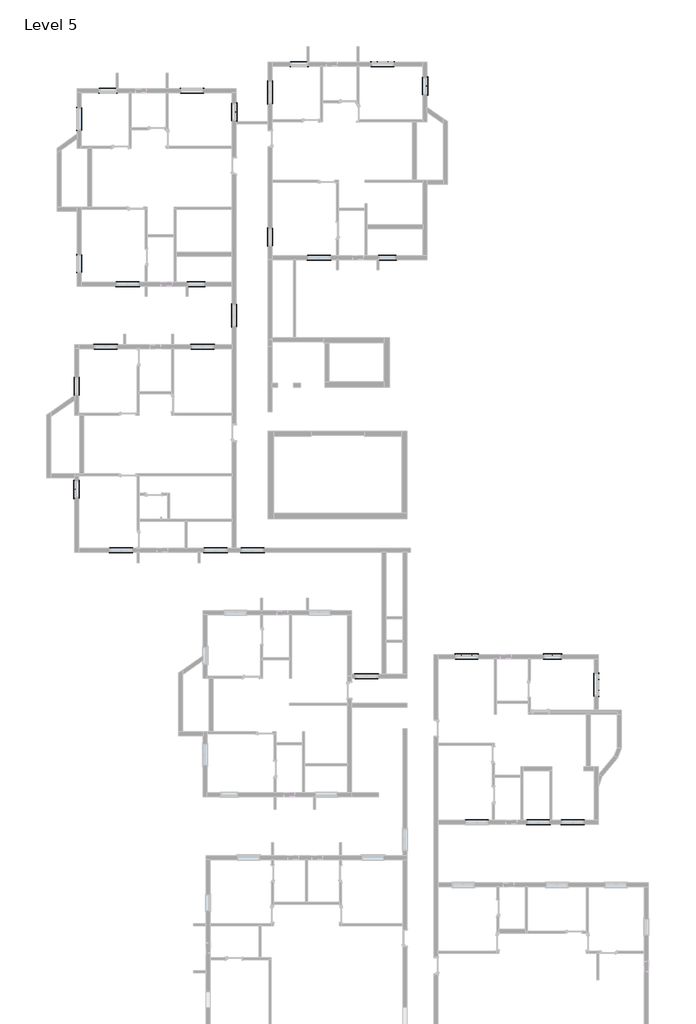
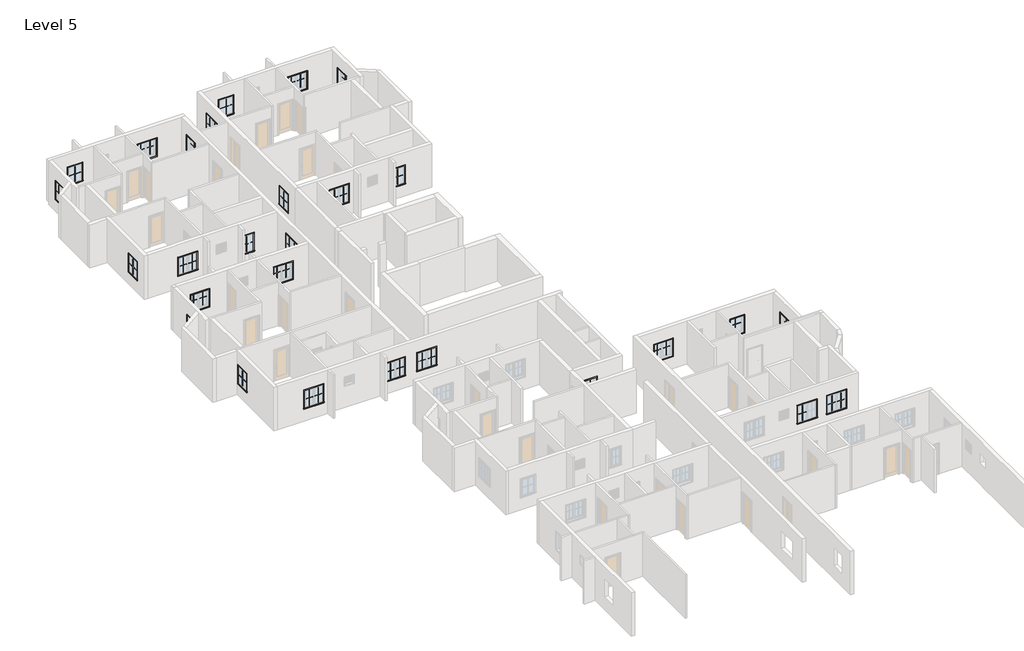
# One storey, part 7 of 7: 101 proxies.
"""IFC4 building model written with IfcOpenShell, lengths in millimetres."""

from ifc_helpers import new_model, si_unit, origin, place, context, project, spatial, transform, mapped, element, save
from components import muntin_pattern_2x2_muntin_pattern_2x2_95b57395, muntin_pattern_2x2_muntin_pattern_2x2_4dfeb3f3, muntin_pattern_2x2_muntin_pattern_2x2_e852a7e4, trim_window_exterior_flat_with_sill_e4b28ec3, trim_window_exterior_flat_with_sill_7cfdd449, trim_window_interior_flat_picture_frame_39ff4276, trim_window_interior_flat_picture_frame_f1e0b15b

model = new_model("IFC4")

# Units and contexts
model_context = context("Model", 3, world=origin())
ifc_project = project(units=[si_unit("LENGTHUNIT", "METRE", prefix="MILLI")], contexts=[model_context])

# Site, building, storey
site = spatial("IfcSite", under=ifc_project)
building = spatial("IfcBuilding", under=site)
storey = spatial("IfcBuildingStorey", under=building, Name="Level 5", Elevation=6400.8)

# Proxies
placement = place(None, origin())
muntin_pattern_2x2_muntin_pattern_2x2_shape = muntin_pattern_2x2_muntin_pattern_2x2_95b57395(model_context)
element("IfcBuildingElementProxy", 1, Name="Muntin Pattern_2x2 : Muntin Pattern_2x2", ObjectType="Muntin Pattern_2x2 : Muntin Pattern_2x2", at=placement, inside=storey, context=model_context, shape_type="MappedRepresentation", body=[
    mapped(muntin_pattern_2x2_muntin_pattern_2x2_shape, transform((-14884.6759469, 4921.5461172, 7385.05), x_axis=(0.0, 1.0, 0.0), y_axis=(-1.0, 0.0, 0.0), z_axis=(0.0, 0.0, 1.0))),
])
element("IfcBuildingElementProxy", 2, Name="Muntin Pattern_2x2 : Muntin Pattern_2x2", ObjectType="Muntin Pattern_2x2 : Muntin Pattern_2x2", at=placement, inside=storey, context=model_context, shape_type="MappedRepresentation", body=[
    mapped(muntin_pattern_2x2_muntin_pattern_2x2_shape, transform((-12990.7362554, 27537.0711172, 7385.05), x_axis=(-1.0, 0.0, 0.0), y_axis=(0.0, -1.0, 0.0), z_axis=(0.0, 0.0, 1.0))),
])
element("IfcBuildingElementProxy", 3, Name="Muntin Pattern_2x2 : Muntin Pattern_2x2", ObjectType="Muntin Pattern_2x2 : Muntin Pattern_2x2", at=placement, inside=storey, context=model_context, shape_type="MappedRepresentation", body=[
    mapped(muntin_pattern_2x2_muntin_pattern_2x2_shape, transform((-5683.5259469, 26431.1755084, 7385.05), x_axis=(0.0, -1.0, 0.0), y_axis=(1.0, 0.0, 0.0), z_axis=(0.0, 0.0, 1.0))),
])
element("IfcBuildingElementProxy", 4, Name="Muntin Pattern_2x2 : Muntin Pattern_2x2", ObjectType="Muntin Pattern_2x2 : Muntin Pattern_2x2", at=placement, inside=storey, context=model_context, shape_type="MappedRepresentation", body=[
    mapped(muntin_pattern_2x2_muntin_pattern_2x2_shape, transform((-7960.0009469, 16513.4711172, 7385.05), x_axis=(-1.0, 0.0, 0.0), y_axis=(0.0, -1.0, 0.0), z_axis=(0.0, 0.0, 1.0))),
])
element("IfcBuildingElementProxy", 5, Name="Muntin Pattern_2x2 : Muntin Pattern_2x2", ObjectType="Muntin Pattern_2x2 : Muntin Pattern_2x2", at=placement, inside=storey, context=model_context, shape_type="MappedRepresentation", body=[
    mapped(muntin_pattern_2x2_muntin_pattern_2x2_shape, transform((-14732.2759469, 17786.6461172, 7385.05), x_axis=(0.0, 1.0, 0.0), y_axis=(-1.0, 0.0, 0.0), z_axis=(0.0, 0.0, 1.0))),
])
element("IfcBuildingElementProxy", 6, Name="Muntin Pattern_2x2 : Muntin Pattern_2x2", ObjectType="Muntin Pattern_2x2 : Muntin Pattern_2x2", at=placement, inside=storey, context=model_context, shape_type="MappedRepresentation", body=[
    mapped(muntin_pattern_2x2_muntin_pattern_2x2_shape, transform((-2075.0862554, 29050.5505084, 7385.05), x_axis=(-1.0, 0.0, 0.0), y_axis=(0.0, -1.0, 0.0), z_axis=(0.0, 0.0, 1.0))),
])
element("IfcBuildingElementProxy", 7, Name="Muntin Pattern_2x2 : Muntin Pattern_2x2", ObjectType="Muntin Pattern_2x2 : Muntin Pattern_2x2", at=placement, inside=storey, context=model_context, shape_type="MappedRepresentation", body=[
    mapped(muntin_pattern_2x2_muntin_pattern_2x2_shape, transform((5213.0740531, 27910.7255084, 7385.05), x_axis=(0.0, -1.0, 0.0), y_axis=(1.0, 0.0, 0.0), z_axis=(0.0, 0.0, 1.0))),
])
element("IfcBuildingElementProxy", 8, Name="Muntin Pattern_2x2 : Muntin Pattern_2x2", ObjectType="Muntin Pattern_2x2 : Muntin Pattern_2x2", at=placement, inside=storey, context=model_context, shape_type="MappedRepresentation", body=[
    mapped(muntin_pattern_2x2_muntin_pattern_2x2_shape, transform((2936.5990531, 18026.9505084, 7385.05), x_axis=(-1.0, 0.0, 0.0), y_axis=(0.0, -1.0, 0.0), z_axis=(0.0, 0.0, 1.0))),
])
element("IfcBuildingElementProxy", 9, Name="Muntin Pattern_2x2 : Muntin Pattern_2x2", ObjectType="Muntin Pattern_2x2 : Muntin Pattern_2x2", at=placement, inside=storey, context=model_context, shape_type="MappedRepresentation", body=[
    mapped(muntin_pattern_2x2_muntin_pattern_2x2_shape, transform((-3835.6759469, 19300.1255084, 7385.05), x_axis=(0.0, 1.0, 0.0), y_axis=(-1.0, 0.0, 0.0), z_axis=(0.0, 0.0, 1.0))),
])
element("IfcBuildingElementProxy", 10, Name="Muntin Pattern_2x2 : Muntin Pattern_2x2", ObjectType="Muntin Pattern_2x2 : Muntin Pattern_2x2", at=placement, inside=storey, context=model_context, shape_type="MappedRepresentation", body=[
    mapped(muntin_pattern_2x2_muntin_pattern_2x2_shape, transform((12366.3490531, -4512.6747229, 7385.05), x_axis=(1.0, 0.0, 0.0), y_axis=(0.0, 1.0, 0.0), z_axis=(0.0, 0.0, 1.0))),
])
element("IfcBuildingElementProxy", 11, Name="Muntin Pattern_2x2 : Muntin Pattern_2x2", ObjectType="Muntin Pattern_2x2 : Muntin Pattern_2x2", at=placement, inside=storey, context=model_context, shape_type="MappedRepresentation", body=[
    mapped(muntin_pattern_2x2_muntin_pattern_2x2_shape, transform((-14675.1259469, 10795.2961172, 7385.05), x_axis=(0.0, -1.0, 0.0), y_axis=(1.0, 0.0, 0.0), z_axis=(0.0, 0.0, 1.0))),
])
muntin_pattern_2x2_muntin_pattern_2x2_2_shape = muntin_pattern_2x2_muntin_pattern_2x2_4dfeb3f3(model_context)
element("IfcBuildingElementProxy", 12, Name="Muntin Pattern_2x2 : Muntin Pattern_2x2", ObjectType="Muntin Pattern_2x2 : Muntin Pattern_2x2", at=placement, inside=storey, context=model_context, shape_type="MappedRepresentation", body=[
    mapped(muntin_pattern_2x2_muntin_pattern_2x2_2_shape, transform((-8498.1634469, 27746.6211172, 7385.05), x_axis=(1.0, 0.0, 0.0), y_axis=(0.0, 1.0, 0.0), z_axis=(0.0, 0.0, 1.0))),
])
element("IfcBuildingElementProxy", 13, Name="Muntin Pattern_2x2 : Muntin Pattern_2x2", ObjectType="Muntin Pattern_2x2 : Muntin Pattern_2x2", at=placement, inside=storey, context=model_context, shape_type="MappedRepresentation", body=[
    mapped(muntin_pattern_2x2_muntin_pattern_2x2_2_shape, transform((-14732.2759469, 25728.9086172, 7385.05), x_axis=(0.0, 1.0, 0.0), y_axis=(-1.0, 0.0, 0.0), z_axis=(0.0, 0.0, 1.0))),
])
element("IfcBuildingElementProxy", 14, Name="Muntin Pattern_2x2 : Muntin Pattern_2x2", ObjectType="Muntin Pattern_2x2 : Muntin Pattern_2x2", at=placement, inside=storey, context=model_context, shape_type="MappedRepresentation", body=[
    mapped(muntin_pattern_2x2_muntin_pattern_2x2_2_shape, transform((-11562.0384469, 16513.4711172, 7385.05), x_axis=(-1.0, 0.0, 0.0), y_axis=(0.0, -1.0, 0.0), z_axis=(0.0, 0.0, 1.0))),
])
element("IfcBuildingElementProxy", 15, Name="Muntin Pattern_2x2 : Muntin Pattern_2x2", ObjectType="Muntin Pattern_2x2 : Muntin Pattern_2x2", at=placement, inside=storey, context=model_context, shape_type="MappedRepresentation", body=[
    mapped(muntin_pattern_2x2_muntin_pattern_2x2_2_shape, transform((-3835.6759469, 27242.3880084, 7385.05), x_axis=(0.0, 1.0, 0.0), y_axis=(-1.0, 0.0, 0.0), z_axis=(0.0, 0.0, 1.0))),
])
element("IfcBuildingElementProxy", 16, Name="Muntin Pattern_2x2 : Muntin Pattern_2x2", ObjectType="Muntin Pattern_2x2 : Muntin Pattern_2x2", at=placement, inside=storey, context=model_context, shape_type="MappedRepresentation", body=[
    mapped(muntin_pattern_2x2_muntin_pattern_2x2_2_shape, transform((2373.0365531, 29260.1005084, 7385.05), x_axis=(1.0, 0.0, 0.0), y_axis=(0.0, 1.0, 0.0), z_axis=(0.0, 0.0, 1.0))),
])
element("IfcBuildingElementProxy", 17, Name="Muntin Pattern_2x2 : Muntin Pattern_2x2", ObjectType="Muntin Pattern_2x2 : Muntin Pattern_2x2", at=placement, inside=storey, context=model_context, shape_type="MappedRepresentation", body=[
    mapped(muntin_pattern_2x2_muntin_pattern_2x2_2_shape, transform((-640.0384469, 18026.9505084, 7385.05), x_axis=(-1.0, 0.0, 0.0), y_axis=(0.0, -1.0, 0.0), z_axis=(0.0, 0.0, 1.0))),
])
element("IfcBuildingElementProxy", 18, Name="Muntin Pattern_2x2 : Muntin Pattern_2x2", ObjectType="Muntin Pattern_2x2 : Muntin Pattern_2x2", at=placement, inside=storey, context=model_context, shape_type="MappedRepresentation", body=[
    mapped(muntin_pattern_2x2_muntin_pattern_2x2_2_shape, transform((14979.3740531, -5923.9622229, 7385.05), x_axis=(0.0, -1.0, 0.0), y_axis=(1.0, 0.0, 0.0), z_axis=(0.0, 0.0, 1.0))),
])
element("IfcBuildingElementProxy", 19, Name="Muntin Pattern_2x2 : Muntin Pattern_2x2", ObjectType="Muntin Pattern_2x2 : Muntin Pattern_2x2", at=placement, inside=storey, context=model_context, shape_type="MappedRepresentation", body=[
    mapped(muntin_pattern_2x2_muntin_pattern_2x2_2_shape, transform((7173.6365531, -4512.6747229, 7385.05), x_axis=(1.0, 0.0, 0.0), y_axis=(0.0, 1.0, 0.0), z_axis=(0.0, 0.0, 1.0))),
])
element("IfcBuildingElementProxy", 20, Name="Muntin Pattern_2x2 : Muntin Pattern_2x2", ObjectType="Muntin Pattern_2x2 : Muntin Pattern_2x2", at=placement, inside=storey, context=model_context, shape_type="MappedRepresentation", body=[
    mapped(muntin_pattern_2x2_muntin_pattern_2x2_2_shape, transform((13825.2615531, -14158.3247229, 7385.05), x_axis=(-1.0, 0.0, 0.0), y_axis=(0.0, -1.0, 0.0), z_axis=(0.0, 0.0, 1.0))),
])
element("IfcBuildingElementProxy", 21, Name="Muntin Pattern_2x2 : Muntin Pattern_2x2", ObjectType="Muntin Pattern_2x2 : Muntin Pattern_2x2", at=placement, inside=storey, context=model_context, shape_type="MappedRepresentation", body=[
    mapped(muntin_pattern_2x2_muntin_pattern_2x2_2_shape, transform((1464.9865531, -5641.6788828, 7385.05), x_axis=(1.0, 0.0, 0.0), y_axis=(0.0, 1.0, 0.0), z_axis=(0.0, 0.0, 1.0))),
])
element("IfcBuildingElementProxy", 22, Name="Muntin Pattern_2x2 : Muntin Pattern_2x2", ObjectType="Muntin Pattern_2x2 : Muntin Pattern_2x2", at=placement, inside=storey, context=model_context, shape_type="MappedRepresentation", body=[
    mapped(muntin_pattern_2x2_muntin_pattern_2x2_2_shape, transform((-4443.6884469, 1349.6711172, 7385.05), x_axis=(-1.0, 0.0, 0.0), y_axis=(0.0, -1.0, 0.0), z_axis=(0.0, 0.0, 1.0))),
])
element("IfcBuildingElementProxy", 23, Name="Muntin Pattern_2x2 : Muntin Pattern_2x2", ObjectType="Muntin Pattern_2x2 : Muntin Pattern_2x2", at=placement, inside=storey, context=model_context, shape_type="MappedRepresentation", body=[
    mapped(muntin_pattern_2x2_muntin_pattern_2x2_2_shape, transform((-6540.8708092, 1349.6711172, 7385.05), x_axis=(-1.0, 0.0, 0.0), y_axis=(0.0, -1.0, 0.0), z_axis=(0.0, 0.0, 1.0))),
])
element("IfcBuildingElementProxy", 24, Name="Muntin Pattern_2x2 : Muntin Pattern_2x2", ObjectType="Muntin Pattern_2x2 : Muntin Pattern_2x2", at=placement, inside=storey, context=model_context, shape_type="MappedRepresentation", body=[
    mapped(muntin_pattern_2x2_muntin_pattern_2x2_2_shape, transform((-11943.0384469, 1349.6711172, 7385.05), x_axis=(-1.0, 0.0, 0.0), y_axis=(0.0, -1.0, 0.0), z_axis=(0.0, 0.0, 1.0))),
])
element("IfcBuildingElementProxy", 25, Name="Muntin Pattern_2x2 : Muntin Pattern_2x2", ObjectType="Muntin Pattern_2x2 : Muntin Pattern_2x2", at=placement, inside=storey, context=model_context, shape_type="MappedRepresentation", body=[
    mapped(muntin_pattern_2x2_muntin_pattern_2x2_2_shape, transform((-13424.2323258, 13141.6211172, 7385.05), x_axis=(1.0, 0.0, 0.0), y_axis=(0.0, 1.0, 0.0), z_axis=(0.0, 0.0, 1.0))),
])
element("IfcBuildingElementProxy", 26, Name="Muntin Pattern_2x2 : Muntin Pattern_2x2", ObjectType="Muntin Pattern_2x2 : Muntin Pattern_2x2", at=placement, inside=storey, context=model_context, shape_type="MappedRepresentation", body=[
    mapped(muntin_pattern_2x2_muntin_pattern_2x2_2_shape, transform((-7888.5634469, 13141.6211172, 7385.05), x_axis=(1.0, 0.0, 0.0), y_axis=(0.0, 1.0, 0.0), z_axis=(0.0, 0.0, 1.0))),
])
element("IfcBuildingElementProxy", 27, Name="Muntin Pattern_2x2 : Muntin Pattern_2x2", ObjectType="Muntin Pattern_2x2 : Muntin Pattern_2x2", at=placement, inside=storey, context=model_context, shape_type="MappedRepresentation", body=[
    mapped(muntin_pattern_2x2_muntin_pattern_2x2_2_shape, transform((-5893.0759469, 14524.3336172, 7385.05), x_axis=(0.0, 1.0, 0.0), y_axis=(-1.0, 0.0, 0.0), z_axis=(0.0, 0.0, 1.0))),
])
muntin_pattern_2x2_muntin_pattern_2x2_3_shape = muntin_pattern_2x2_muntin_pattern_2x2_e852a7e4(model_context)
element("IfcBuildingElementProxy", 28, Name="Muntin Pattern_2x2 : Muntin Pattern_2x2", ObjectType="Muntin Pattern_2x2 : Muntin Pattern_2x2", at=placement, inside=storey, context=model_context, shape_type="MappedRepresentation", body=[
    mapped(muntin_pattern_2x2_muntin_pattern_2x2_3_shape, transform((-7891.7384469, 27746.6211172, 7385.05), x_axis=(-1.0, 0.0, 0.0), y_axis=(0.0, -1.0, 0.0), z_axis=(0.0, 0.0, 1.0))),
])
element("IfcBuildingElementProxy", 29, Name="Muntin Pattern_2x2 : Muntin Pattern_2x2", ObjectType="Muntin Pattern_2x2 : Muntin Pattern_2x2", at=placement, inside=storey, context=model_context, shape_type="MappedRepresentation", body=[
    mapped(muntin_pattern_2x2_muntin_pattern_2x2_3_shape, transform((-14732.2759469, 26335.3336172, 7385.05), x_axis=(0.0, -1.0, 0.0), y_axis=(1.0, 0.0, 0.0), z_axis=(0.0, 0.0, 1.0))),
])
element("IfcBuildingElementProxy", 30, Name="Muntin Pattern_2x2 : Muntin Pattern_2x2", ObjectType="Muntin Pattern_2x2 : Muntin Pattern_2x2", at=placement, inside=storey, context=model_context, shape_type="MappedRepresentation", body=[
    mapped(muntin_pattern_2x2_muntin_pattern_2x2_3_shape, transform((-12168.4634469, 16513.4711172, 7385.05), x_axis=(1.0, 0.0, 0.0), y_axis=(0.0, 1.0, 0.0), z_axis=(0.0, 0.0, 1.0))),
])
element("IfcBuildingElementProxy", 31, Name="Muntin Pattern_2x2 : Muntin Pattern_2x2", ObjectType="Muntin Pattern_2x2 : Muntin Pattern_2x2", at=placement, inside=storey, context=model_context, shape_type="MappedRepresentation", body=[
    mapped(muntin_pattern_2x2_muntin_pattern_2x2_3_shape, transform((-3835.6759469, 27848.8130084, 7385.05), x_axis=(0.0, -1.0, 0.0), y_axis=(1.0, 0.0, 0.0), z_axis=(0.0, 0.0, 1.0))),
])
element("IfcBuildingElementProxy", 32, Name="Muntin Pattern_2x2 : Muntin Pattern_2x2", ObjectType="Muntin Pattern_2x2 : Muntin Pattern_2x2", at=placement, inside=storey, context=model_context, shape_type="MappedRepresentation", body=[
    mapped(muntin_pattern_2x2_muntin_pattern_2x2_3_shape, transform((2979.4615531, 29260.1005084, 7385.05), x_axis=(-1.0, 0.0, 0.0), y_axis=(0.0, -1.0, 0.0), z_axis=(0.0, 0.0, 1.0))),
])
element("IfcBuildingElementProxy", 33, Name="Muntin Pattern_2x2 : Muntin Pattern_2x2", ObjectType="Muntin Pattern_2x2 : Muntin Pattern_2x2", at=placement, inside=storey, context=model_context, shape_type="MappedRepresentation", body=[
    mapped(muntin_pattern_2x2_muntin_pattern_2x2_3_shape, transform((-1246.4634469, 18026.9505084, 7385.05), x_axis=(1.0, 0.0, 0.0), y_axis=(0.0, 1.0, 0.0), z_axis=(0.0, 0.0, 1.0))),
])
element("IfcBuildingElementProxy", 34, Name="Muntin Pattern_2x2 : Muntin Pattern_2x2", ObjectType="Muntin Pattern_2x2 : Muntin Pattern_2x2", at=placement, inside=storey, context=model_context, shape_type="MappedRepresentation", body=[
    mapped(muntin_pattern_2x2_muntin_pattern_2x2_3_shape, transform((14979.3740531, -6530.3872229, 7385.05), x_axis=(0.0, 1.0, 0.0), y_axis=(-1.0, 0.0, 0.0), z_axis=(0.0, 0.0, 1.0))),
])
element("IfcBuildingElementProxy", 35, Name="Muntin Pattern_2x2 : Muntin Pattern_2x2", ObjectType="Muntin Pattern_2x2 : Muntin Pattern_2x2", at=placement, inside=storey, context=model_context, shape_type="MappedRepresentation", body=[
    mapped(muntin_pattern_2x2_muntin_pattern_2x2_3_shape, transform((7780.0615531, -4512.6747229, 7385.05), x_axis=(-1.0, 0.0, 0.0), y_axis=(0.0, -1.0, 0.0), z_axis=(0.0, 0.0, 1.0))),
])
element("IfcBuildingElementProxy", 36, Name="Muntin Pattern_2x2 : Muntin Pattern_2x2", ObjectType="Muntin Pattern_2x2 : Muntin Pattern_2x2", at=placement, inside=storey, context=model_context, shape_type="MappedRepresentation", body=[
    mapped(muntin_pattern_2x2_muntin_pattern_2x2_3_shape, transform((13218.8365531, -14158.3247229, 7385.05), x_axis=(1.0, 0.0, 0.0), y_axis=(0.0, 1.0, 0.0), z_axis=(0.0, 0.0, 1.0))),
])
element("IfcBuildingElementProxy", 37, Name="Muntin Pattern_2x2 : Muntin Pattern_2x2", ObjectType="Muntin Pattern_2x2 : Muntin Pattern_2x2", at=placement, inside=storey, context=model_context, shape_type="MappedRepresentation", body=[
    mapped(muntin_pattern_2x2_muntin_pattern_2x2_3_shape, transform((11263.0365531, -14158.3247229, 7385.05), x_axis=(1.0, 0.0, 0.0), y_axis=(0.0, 1.0, 0.0), z_axis=(0.0, 0.0, 1.0))),
])
element("IfcBuildingElementProxy", 38, Name="Muntin Pattern_2x2 : Muntin Pattern_2x2", ObjectType="Muntin Pattern_2x2 : Muntin Pattern_2x2", at=placement, inside=storey, context=model_context, shape_type="MappedRepresentation", body=[
    mapped(muntin_pattern_2x2_muntin_pattern_2x2_3_shape, transform((2071.4115531, -5641.6788828, 7385.05), x_axis=(-1.0, 0.0, 0.0), y_axis=(0.0, -1.0, 0.0), z_axis=(0.0, 0.0, 1.0))),
])
element("IfcBuildingElementProxy", 39, Name="Muntin Pattern_2x2 : Muntin Pattern_2x2", ObjectType="Muntin Pattern_2x2 : Muntin Pattern_2x2", at=placement, inside=storey, context=model_context, shape_type="MappedRepresentation", body=[
    mapped(muntin_pattern_2x2_muntin_pattern_2x2_3_shape, transform((-5050.1134469, 1349.6711172, 7385.05), x_axis=(1.0, 0.0, 0.0), y_axis=(0.0, 1.0, 0.0), z_axis=(0.0, 0.0, 1.0))),
])
element("IfcBuildingElementProxy", 40, Name="Muntin Pattern_2x2 : Muntin Pattern_2x2", ObjectType="Muntin Pattern_2x2 : Muntin Pattern_2x2", at=placement, inside=storey, context=model_context, shape_type="MappedRepresentation", body=[
    mapped(muntin_pattern_2x2_muntin_pattern_2x2_3_shape, transform((-7147.2958092, 1349.6711172, 7385.05), x_axis=(1.0, 0.0, 0.0), y_axis=(0.0, 1.0, 0.0), z_axis=(0.0, 0.0, 1.0))),
])
element("IfcBuildingElementProxy", 41, Name="Muntin Pattern_2x2 : Muntin Pattern_2x2", ObjectType="Muntin Pattern_2x2 : Muntin Pattern_2x2", at=placement, inside=storey, context=model_context, shape_type="MappedRepresentation", body=[
    mapped(muntin_pattern_2x2_muntin_pattern_2x2_3_shape, transform((-12549.4634469, 1349.6711172, 7385.05), x_axis=(1.0, 0.0, 0.0), y_axis=(0.0, 1.0, 0.0), z_axis=(0.0, 0.0, 1.0))),
])
element("IfcBuildingElementProxy", 42, Name="Muntin Pattern_2x2 : Muntin Pattern_2x2", ObjectType="Muntin Pattern_2x2 : Muntin Pattern_2x2", at=placement, inside=storey, context=model_context, shape_type="MappedRepresentation", body=[
    mapped(muntin_pattern_2x2_muntin_pattern_2x2_3_shape, transform((-12817.8073258, 13141.6211172, 7385.05), x_axis=(-1.0, 0.0, 0.0), y_axis=(0.0, -1.0, 0.0), z_axis=(0.0, 0.0, 1.0))),
])
element("IfcBuildingElementProxy", 43, Name="Muntin Pattern_2x2 : Muntin Pattern_2x2", ObjectType="Muntin Pattern_2x2 : Muntin Pattern_2x2", at=placement, inside=storey, context=model_context, shape_type="MappedRepresentation", body=[
    mapped(muntin_pattern_2x2_muntin_pattern_2x2_3_shape, transform((-7282.1384469, 13141.6211172, 7385.05), x_axis=(-1.0, 0.0, 0.0), y_axis=(0.0, -1.0, 0.0), z_axis=(0.0, 0.0, 1.0))),
])
element("IfcBuildingElementProxy", 44, Name="Muntin Pattern_2x2 : Muntin Pattern_2x2", ObjectType="Muntin Pattern_2x2 : Muntin Pattern_2x2", at=placement, inside=storey, context=model_context, shape_type="MappedRepresentation", body=[
    mapped(muntin_pattern_2x2_muntin_pattern_2x2_3_shape, transform((-5893.0759469, 15130.7586172, 7385.05), x_axis=(0.0, -1.0, 0.0), y_axis=(1.0, 0.0, 0.0), z_axis=(0.0, 0.0, 1.0))),
])
trim_window_exterior_flat_with_sill_shape = trim_window_exterior_flat_with_sill_e4b28ec3(model_context)
element("IfcBuildingElementProxy", 45, Name="Trim-Window-Exterior-Flat : with Sill", ObjectType="Trim-Window-Exterior-Flat : with Sill", at=placement, inside=storey, context=model_context, shape_type="MappedRepresentation", body=[
    mapped(trim_window_exterior_flat_with_sill_shape, transform((-14894.2009469, 4921.5461172, 8534.4), x_axis=(0.0, -1.0, 0.0), y_axis=(0.0, 0.0, 1.0), z_axis=(-1.0, 0.0, 0.0))),
])
element("IfcBuildingElementProxy", 46, Name="Trim-Window-Exterior-Flat : with Sill", ObjectType="Trim-Window-Exterior-Flat : with Sill", at=placement, inside=storey, context=model_context, shape_type="MappedRepresentation", body=[
    mapped(trim_window_exterior_flat_with_sill_shape, transform((-12990.7362554, 27527.5461172, 8534.4), x_axis=(1.0, 0.0, 0.0), y_axis=(0.0, 0.0, 1.0), z_axis=(0.0, -1.0, 0.0))),
])
element("IfcBuildingElementProxy", 47, Name="Trim-Window-Exterior-Flat : with Sill", ObjectType="Trim-Window-Exterior-Flat : with Sill", at=placement, inside=storey, context=model_context, shape_type="MappedRepresentation", body=[
    mapped(trim_window_exterior_flat_with_sill_shape, transform((-5674.0009469, 26431.1755084, 8534.4), x_axis=(0.0, 1.0, 0.0), y_axis=(0.0, 0.0, 1.0), z_axis=(1.0, 0.0, 0.0))),
])
element("IfcBuildingElementProxy", 48, Name="Trim-Window-Exterior-Flat : with Sill", ObjectType="Trim-Window-Exterior-Flat : with Sill", at=placement, inside=storey, context=model_context, shape_type="MappedRepresentation", body=[
    mapped(trim_window_exterior_flat_with_sill_shape, transform((-7960.0009469, 16503.9461172, 8534.4), x_axis=(1.0, 0.0, 0.0), y_axis=(0.0, 0.0, 1.0), z_axis=(0.0, -1.0, 0.0))),
])
element("IfcBuildingElementProxy", 49, Name="Trim-Window-Exterior-Flat : with Sill", ObjectType="Trim-Window-Exterior-Flat : with Sill", at=placement, inside=storey, context=model_context, shape_type="MappedRepresentation", body=[
    mapped(trim_window_exterior_flat_with_sill_shape, transform((-14741.8009469, 17786.6461172, 8534.4), x_axis=(0.0, -1.0, 0.0), y_axis=(0.0, 0.0, 1.0), z_axis=(-1.0, 0.0, 0.0))),
])
element("IfcBuildingElementProxy", 50, Name="Trim-Window-Exterior-Flat : with Sill", ObjectType="Trim-Window-Exterior-Flat : with Sill", at=placement, inside=storey, context=model_context, shape_type="MappedRepresentation", body=[
    mapped(trim_window_exterior_flat_with_sill_shape, transform((-2075.0862554, 29041.0255084, 8534.4), x_axis=(1.0, 0.0, 0.0), y_axis=(0.0, 0.0, 1.0), z_axis=(0.0, -1.0, 0.0))),
])
element("IfcBuildingElementProxy", 51, Name="Trim-Window-Exterior-Flat : with Sill", ObjectType="Trim-Window-Exterior-Flat : with Sill", at=placement, inside=storey, context=model_context, shape_type="MappedRepresentation", body=[
    mapped(trim_window_exterior_flat_with_sill_shape, transform((5222.5990531, 27910.7255084, 8534.4), x_axis=(0.0, 1.0, 0.0), y_axis=(0.0, 0.0, 1.0), z_axis=(1.0, 0.0, 0.0))),
])
element("IfcBuildingElementProxy", 52, Name="Trim-Window-Exterior-Flat : with Sill", ObjectType="Trim-Window-Exterior-Flat : with Sill", at=placement, inside=storey, context=model_context, shape_type="MappedRepresentation", body=[
    mapped(trim_window_exterior_flat_with_sill_shape, transform((2936.5990531, 18017.4255084, 8534.4), x_axis=(1.0, 0.0, 0.0), y_axis=(0.0, 0.0, 1.0), z_axis=(0.0, -1.0, 0.0))),
])
element("IfcBuildingElementProxy", 53, Name="Trim-Window-Exterior-Flat : with Sill", ObjectType="Trim-Window-Exterior-Flat : with Sill", at=placement, inside=storey, context=model_context, shape_type="MappedRepresentation", body=[
    mapped(trim_window_exterior_flat_with_sill_shape, transform((-3845.2009469, 19300.1255084, 8534.4), x_axis=(0.0, -1.0, 0.0), y_axis=(0.0, 0.0, 1.0), z_axis=(-1.0, 0.0, 0.0))),
])
element("IfcBuildingElementProxy", 54, Name="Trim-Window-Exterior-Flat : with Sill", ObjectType="Trim-Window-Exterior-Flat : with Sill", at=placement, inside=storey, context=model_context, shape_type="MappedRepresentation", body=[
    mapped(trim_window_exterior_flat_with_sill_shape, transform((12366.3490531, -4503.1497229, 8534.4), x_axis=(-1.0, 0.0, 0.0), y_axis=(0.0, 0.0, 1.0), z_axis=(0.0, 1.0, 0.0))),
])
element("IfcBuildingElementProxy", 55, Name="Trim-Window-Exterior-Flat : with Sill", ObjectType="Trim-Window-Exterior-Flat : with Sill", at=placement, inside=storey, context=model_context, shape_type="MappedRepresentation", body=[
    mapped(trim_window_exterior_flat_with_sill_shape, transform((-14665.6009469, 10795.2961172, 8534.4), x_axis=(0.0, 1.0, 0.0), y_axis=(0.0, 0.0, 1.0), z_axis=(1.0, 0.0, 0.0))),
])
trim_window_exterior_flat_with_sill_2_shape = trim_window_exterior_flat_with_sill_7cfdd449(model_context)
element("IfcBuildingElementProxy", 56, Name="Trim-Window-Exterior-Flat : with Sill", ObjectType="Trim-Window-Exterior-Flat : with Sill", at=placement, inside=storey, context=model_context, shape_type="MappedRepresentation", body=[
    mapped(trim_window_exterior_flat_with_sill_2_shape, transform((-8194.9509469, 27756.1461172, 8534.4), x_axis=(-1.0, 0.0, 0.0), y_axis=(0.0, 0.0, 1.0), z_axis=(0.0, 1.0, 0.0))),
])
element("IfcBuildingElementProxy", 57, Name="Trim-Window-Exterior-Flat : with Sill", ObjectType="Trim-Window-Exterior-Flat : with Sill", at=placement, inside=storey, context=model_context, shape_type="MappedRepresentation", body=[
    mapped(trim_window_exterior_flat_with_sill_2_shape, transform((-14741.8009469, 26032.1211172, 8534.4), x_axis=(0.0, -1.0, 0.0), y_axis=(0.0, 0.0, 1.0), z_axis=(-1.0, 0.0, 0.0))),
])
element("IfcBuildingElementProxy", 58, Name="Trim-Window-Exterior-Flat : with Sill", ObjectType="Trim-Window-Exterior-Flat : with Sill", at=placement, inside=storey, context=model_context, shape_type="MappedRepresentation", body=[
    mapped(trim_window_exterior_flat_with_sill_2_shape, transform((-11865.2509469, 16503.9461172, 8534.4), x_axis=(1.0, 0.0, 0.0), y_axis=(0.0, 0.0, 1.0), z_axis=(0.0, -1.0, 0.0))),
])
element("IfcBuildingElementProxy", 59, Name="Trim-Window-Exterior-Flat : with Sill", ObjectType="Trim-Window-Exterior-Flat : with Sill", at=placement, inside=storey, context=model_context, shape_type="MappedRepresentation", body=[
    mapped(trim_window_exterior_flat_with_sill_2_shape, transform((-3845.2009469, 27545.6005084, 8534.4), x_axis=(0.0, -1.0, 0.0), y_axis=(0.0, 0.0, 1.0), z_axis=(-1.0, 0.0, 0.0))),
])
element("IfcBuildingElementProxy", 60, Name="Trim-Window-Exterior-Flat : with Sill", ObjectType="Trim-Window-Exterior-Flat : with Sill", at=placement, inside=storey, context=model_context, shape_type="MappedRepresentation", body=[
    mapped(trim_window_exterior_flat_with_sill_2_shape, transform((2676.2490531, 29269.6255084, 8534.4), x_axis=(-1.0, 0.0, 0.0), y_axis=(0.0, 0.0, 1.0), z_axis=(0.0, 1.0, 0.0))),
])
element("IfcBuildingElementProxy", 61, Name="Trim-Window-Exterior-Flat : with Sill", ObjectType="Trim-Window-Exterior-Flat : with Sill", at=placement, inside=storey, context=model_context, shape_type="MappedRepresentation", body=[
    mapped(trim_window_exterior_flat_with_sill_2_shape, transform((-943.2509469, 18017.4255084, 8534.4), x_axis=(1.0, 0.0, 0.0), y_axis=(0.0, 0.0, 1.0), z_axis=(0.0, -1.0, 0.0))),
])
element("IfcBuildingElementProxy", 62, Name="Trim-Window-Exterior-Flat : with Sill", ObjectType="Trim-Window-Exterior-Flat : with Sill", at=placement, inside=storey, context=model_context, shape_type="MappedRepresentation", body=[
    mapped(trim_window_exterior_flat_with_sill_2_shape, transform((14988.8990531, -6227.1747229, 8534.4), x_axis=(0.0, 1.0, 0.0), y_axis=(0.0, 0.0, 1.0), z_axis=(1.0, 0.0, 0.0))),
])
element("IfcBuildingElementProxy", 63, Name="Trim-Window-Exterior-Flat : with Sill", ObjectType="Trim-Window-Exterior-Flat : with Sill", at=placement, inside=storey, context=model_context, shape_type="MappedRepresentation", body=[
    mapped(trim_window_exterior_flat_with_sill_2_shape, transform((7476.8490531, -4503.1497229, 8534.4), x_axis=(-1.0, 0.0, 0.0), y_axis=(0.0, 0.0, 1.0), z_axis=(0.0, 1.0, 0.0))),
])
element("IfcBuildingElementProxy", 64, Name="Trim-Window-Exterior-Flat : with Sill", ObjectType="Trim-Window-Exterior-Flat : with Sill", at=placement, inside=storey, context=model_context, shape_type="MappedRepresentation", body=[
    mapped(trim_window_exterior_flat_with_sill_2_shape, transform((13522.0490531, -14167.8497229, 8534.4), x_axis=(1.0, 0.0, 0.0), y_axis=(0.0, 0.0, 1.0), z_axis=(0.0, -1.0, 0.0))),
])
element("IfcBuildingElementProxy", 65, Name="Trim-Window-Exterior-Flat : with Sill", ObjectType="Trim-Window-Exterior-Flat : with Sill", at=placement, inside=storey, context=model_context, shape_type="MappedRepresentation", body=[
    mapped(trim_window_exterior_flat_with_sill_2_shape, transform((11566.2490531, -14167.8497229, 8534.4), x_axis=(1.0, 0.0, 0.0), y_axis=(0.0, 0.0, 1.0), z_axis=(0.0, -1.0, 0.0))),
])
element("IfcBuildingElementProxy", 66, Name="Trim-Window-Exterior-Flat : with Sill", ObjectType="Trim-Window-Exterior-Flat : with Sill", at=placement, inside=storey, context=model_context, shape_type="MappedRepresentation", body=[
    mapped(trim_window_exterior_flat_with_sill_2_shape, transform((1768.1990531, -5632.1538828, 8534.4), x_axis=(-1.0, 0.0, 0.0), y_axis=(0.0, 0.0, 1.0), z_axis=(0.0, 1.0, 0.0))),
])
element("IfcBuildingElementProxy", 67, Name="Trim-Window-Exterior-Flat : with Sill", ObjectType="Trim-Window-Exterior-Flat : with Sill", at=placement, inside=storey, context=model_context, shape_type="MappedRepresentation", body=[
    mapped(trim_window_exterior_flat_with_sill_2_shape, transform((-4746.9009469, 1340.1461172, 8534.4), x_axis=(1.0, 0.0, 0.0), y_axis=(0.0, 0.0, 1.0), z_axis=(0.0, -1.0, 0.0))),
])
element("IfcBuildingElementProxy", 68, Name="Trim-Window-Exterior-Flat : with Sill", ObjectType="Trim-Window-Exterior-Flat : with Sill", at=placement, inside=storey, context=model_context, shape_type="MappedRepresentation", body=[
    mapped(trim_window_exterior_flat_with_sill_2_shape, transform((-6844.0833092, 1340.1461172, 8534.4), x_axis=(1.0, 0.0, 0.0), y_axis=(0.0, 0.0, 1.0), z_axis=(0.0, -1.0, 0.0))),
])
element("IfcBuildingElementProxy", 69, Name="Trim-Window-Exterior-Flat : with Sill", ObjectType="Trim-Window-Exterior-Flat : with Sill", at=placement, inside=storey, context=model_context, shape_type="MappedRepresentation", body=[
    mapped(trim_window_exterior_flat_with_sill_2_shape, transform((-12246.2509469, 1340.1461172, 8534.4), x_axis=(1.0, 0.0, 0.0), y_axis=(0.0, 0.0, 1.0), z_axis=(0.0, -1.0, 0.0))),
])
element("IfcBuildingElementProxy", 70, Name="Trim-Window-Exterior-Flat : with Sill", ObjectType="Trim-Window-Exterior-Flat : with Sill", at=placement, inside=storey, context=model_context, shape_type="MappedRepresentation", body=[
    mapped(trim_window_exterior_flat_with_sill_2_shape, transform((-13121.0198258, 13151.1461172, 8534.4), x_axis=(-1.0, 0.0, 0.0), y_axis=(0.0, 0.0, 1.0), z_axis=(0.0, 1.0, 0.0))),
])
element("IfcBuildingElementProxy", 71, Name="Trim-Window-Exterior-Flat : with Sill", ObjectType="Trim-Window-Exterior-Flat : with Sill", at=placement, inside=storey, context=model_context, shape_type="MappedRepresentation", body=[
    mapped(trim_window_exterior_flat_with_sill_2_shape, transform((-7585.3509469, 13151.1461172, 8534.4), x_axis=(-1.0, 0.0, 0.0), y_axis=(0.0, 0.0, 1.0), z_axis=(0.0, 1.0, 0.0))),
])
element("IfcBuildingElementProxy", 72, Name="Trim-Window-Exterior-Flat : with Sill", ObjectType="Trim-Window-Exterior-Flat : with Sill", at=placement, inside=storey, context=model_context, shape_type="MappedRepresentation", body=[
    mapped(trim_window_exterior_flat_with_sill_2_shape, transform((-5902.6009469, 14827.5461172, 8534.4), x_axis=(0.0, -1.0, 0.0), y_axis=(0.0, 0.0, 1.0), z_axis=(-1.0, 0.0, 0.0))),
])
trim_window_interior_flat_picture_frame_shape = trim_window_interior_flat_picture_frame_39ff4276(model_context)
element("IfcBuildingElementProxy", 73, Name="Trim-Window-Interior-Flat : Picture Frame", ObjectType="Trim-Window-Interior-Flat : Picture Frame", at=placement, inside=storey, context=model_context, shape_type="MappedRepresentation", body=[
    mapped(trim_window_interior_flat_picture_frame_shape, transform((-14665.6009469, 4921.5461172, 8534.4), x_axis=(0.0, 1.0, 0.0), y_axis=(0.0, 0.0, 1.0), z_axis=(1.0, 0.0, 0.0))),
])
element("IfcBuildingElementProxy", 74, Name="Trim-Window-Interior-Flat : Picture Frame", ObjectType="Trim-Window-Interior-Flat : Picture Frame", at=placement, inside=storey, context=model_context, shape_type="MappedRepresentation", body=[
    mapped(trim_window_interior_flat_picture_frame_shape, transform((-12990.7362554, 27756.1461172, 8534.4), x_axis=(-1.0, 0.0, 0.0), y_axis=(0.0, 0.0, 1.0), z_axis=(0.0, 1.0, 0.0))),
])
element("IfcBuildingElementProxy", 75, Name="Trim-Window-Interior-Flat : Picture Frame", ObjectType="Trim-Window-Interior-Flat : Picture Frame", at=placement, inside=storey, context=model_context, shape_type="MappedRepresentation", body=[
    mapped(trim_window_interior_flat_picture_frame_shape, transform((-5902.6009469, 26431.1755084, 8534.4), x_axis=(0.0, -1.0, 0.0), y_axis=(0.0, 0.0, 1.0), z_axis=(-1.0, 0.0, 0.0))),
])
element("IfcBuildingElementProxy", 76, Name="Trim-Window-Interior-Flat : Picture Frame", ObjectType="Trim-Window-Interior-Flat : Picture Frame", at=placement, inside=storey, context=model_context, shape_type="MappedRepresentation", body=[
    mapped(trim_window_interior_flat_picture_frame_shape, transform((-7960.0009469, 16732.5461172, 8534.4), x_axis=(-1.0, 0.0, 0.0), y_axis=(0.0, 0.0, 1.0), z_axis=(0.0, 1.0, 0.0))),
])
element("IfcBuildingElementProxy", 77, Name="Trim-Window-Interior-Flat : Picture Frame", ObjectType="Trim-Window-Interior-Flat : Picture Frame", at=placement, inside=storey, context=model_context, shape_type="MappedRepresentation", body=[
    mapped(trim_window_interior_flat_picture_frame_shape, transform((-14513.2009469, 17786.6461172, 8534.4), x_axis=(0.0, 1.0, 0.0), y_axis=(0.0, 0.0, 1.0), z_axis=(1.0, 0.0, 0.0))),
])
element("IfcBuildingElementProxy", 78, Name="Trim-Window-Interior-Flat : Picture Frame", ObjectType="Trim-Window-Interior-Flat : Picture Frame", at=placement, inside=storey, context=model_context, shape_type="MappedRepresentation", body=[
    mapped(trim_window_interior_flat_picture_frame_shape, transform((-2075.0862554, 29269.6255084, 8534.4), x_axis=(-1.0, 0.0, 0.0), y_axis=(0.0, 0.0, 1.0), z_axis=(0.0, 1.0, 0.0))),
])
element("IfcBuildingElementProxy", 79, Name="Trim-Window-Interior-Flat : Picture Frame", ObjectType="Trim-Window-Interior-Flat : Picture Frame", at=placement, inside=storey, context=model_context, shape_type="MappedRepresentation", body=[
    mapped(trim_window_interior_flat_picture_frame_shape, transform((4993.9990531, 27910.7255084, 8534.4), x_axis=(0.0, -1.0, 0.0), y_axis=(0.0, 0.0, 1.0), z_axis=(-1.0, 0.0, 0.0))),
])
element("IfcBuildingElementProxy", 80, Name="Trim-Window-Interior-Flat : Picture Frame", ObjectType="Trim-Window-Interior-Flat : Picture Frame", at=placement, inside=storey, context=model_context, shape_type="MappedRepresentation", body=[
    mapped(trim_window_interior_flat_picture_frame_shape, transform((2936.5990531, 18246.0255084, 8534.4), x_axis=(-1.0, 0.0, 0.0), y_axis=(0.0, 0.0, 1.0), z_axis=(0.0, 1.0, 0.0))),
])
element("IfcBuildingElementProxy", 81, Name="Trim-Window-Interior-Flat : Picture Frame", ObjectType="Trim-Window-Interior-Flat : Picture Frame", at=placement, inside=storey, context=model_context, shape_type="MappedRepresentation", body=[
    mapped(trim_window_interior_flat_picture_frame_shape, transform((-3616.6009469, 19300.1255084, 8534.4), x_axis=(0.0, 1.0, 0.0), y_axis=(0.0, 0.0, 1.0), z_axis=(1.0, 0.0, 0.0))),
])
element("IfcBuildingElementProxy", 82, Name="Trim-Window-Interior-Flat : Picture Frame", ObjectType="Trim-Window-Interior-Flat : Picture Frame", at=placement, inside=storey, context=model_context, shape_type="MappedRepresentation", body=[
    mapped(trim_window_interior_flat_picture_frame_shape, transform((12366.3490531, -4731.7497229, 8534.4), x_axis=(1.0, 0.0, 0.0), y_axis=(0.0, 0.0, 1.0), z_axis=(0.0, -1.0, 0.0))),
])
element("IfcBuildingElementProxy", 83, Name="Trim-Window-Interior-Flat : Picture Frame", ObjectType="Trim-Window-Interior-Flat : Picture Frame", at=placement, inside=storey, context=model_context, shape_type="MappedRepresentation", body=[
    mapped(trim_window_interior_flat_picture_frame_shape, transform((-14894.2009469, 10795.2961172, 8534.4), x_axis=(0.0, -1.0, 0.0), y_axis=(0.0, 0.0, 1.0), z_axis=(-1.0, 0.0, 0.0))),
])
trim_window_interior_flat_picture_frame_2_shape = trim_window_interior_flat_picture_frame_f1e0b15b(model_context)
element("IfcBuildingElementProxy", 84, Name="Trim-Window-Interior-Flat : Picture Frame", ObjectType="Trim-Window-Interior-Flat : Picture Frame", at=placement, inside=storey, context=model_context, shape_type="MappedRepresentation", body=[
    mapped(trim_window_interior_flat_picture_frame_2_shape, transform((-8194.9509469, 27527.5461172, 8534.4), x_axis=(1.0, 0.0, 0.0), y_axis=(0.0, 0.0, 1.0), z_axis=(0.0, -1.0, 0.0))),
])
element("IfcBuildingElementProxy", 85, Name="Trim-Window-Interior-Flat : Picture Frame", ObjectType="Trim-Window-Interior-Flat : Picture Frame", at=placement, inside=storey, context=model_context, shape_type="MappedRepresentation", body=[
    mapped(trim_window_interior_flat_picture_frame_2_shape, transform((-14513.2009469, 26032.1211172, 8534.4), x_axis=(0.0, 1.0, 0.0), y_axis=(0.0, 0.0, 1.0), z_axis=(1.0, 0.0, 0.0))),
])
element("IfcBuildingElementProxy", 86, Name="Trim-Window-Interior-Flat : Picture Frame", ObjectType="Trim-Window-Interior-Flat : Picture Frame", at=placement, inside=storey, context=model_context, shape_type="MappedRepresentation", body=[
    mapped(trim_window_interior_flat_picture_frame_2_shape, transform((-11865.2509469, 16732.5461172, 8534.4), x_axis=(-1.0, 0.0, 0.0), y_axis=(0.0, 0.0, 1.0), z_axis=(0.0, 1.0, 0.0))),
])
element("IfcBuildingElementProxy", 87, Name="Trim-Window-Interior-Flat : Picture Frame", ObjectType="Trim-Window-Interior-Flat : Picture Frame", at=placement, inside=storey, context=model_context, shape_type="MappedRepresentation", body=[
    mapped(trim_window_interior_flat_picture_frame_2_shape, transform((-3616.6009469, 27545.6005084, 8534.4), x_axis=(0.0, 1.0, 0.0), y_axis=(0.0, 0.0, 1.0), z_axis=(1.0, 0.0, 0.0))),
])
element("IfcBuildingElementProxy", 88, Name="Trim-Window-Interior-Flat : Picture Frame", ObjectType="Trim-Window-Interior-Flat : Picture Frame", at=placement, inside=storey, context=model_context, shape_type="MappedRepresentation", body=[
    mapped(trim_window_interior_flat_picture_frame_2_shape, transform((2676.2490531, 29041.0255084, 8534.4), x_axis=(1.0, 0.0, 0.0), y_axis=(0.0, 0.0, 1.0), z_axis=(0.0, -1.0, 0.0))),
])
element("IfcBuildingElementProxy", 89, Name="Trim-Window-Interior-Flat : Picture Frame", ObjectType="Trim-Window-Interior-Flat : Picture Frame", at=placement, inside=storey, context=model_context, shape_type="MappedRepresentation", body=[
    mapped(trim_window_interior_flat_picture_frame_2_shape, transform((-943.2509469, 18246.0255084, 8534.4), x_axis=(-1.0, 0.0, 0.0), y_axis=(0.0, 0.0, 1.0), z_axis=(0.0, 1.0, 0.0))),
])
element("IfcBuildingElementProxy", 90, Name="Trim-Window-Interior-Flat : Picture Frame", ObjectType="Trim-Window-Interior-Flat : Picture Frame", at=placement, inside=storey, context=model_context, shape_type="MappedRepresentation", body=[
    mapped(trim_window_interior_flat_picture_frame_2_shape, transform((14760.2990531, -6227.1747229, 8534.4), x_axis=(0.0, -1.0, 0.0), y_axis=(0.0, 0.0, 1.0), z_axis=(-1.0, 0.0, 0.0))),
])
element("IfcBuildingElementProxy", 91, Name="Trim-Window-Interior-Flat : Picture Frame", ObjectType="Trim-Window-Interior-Flat : Picture Frame", at=placement, inside=storey, context=model_context, shape_type="MappedRepresentation", body=[
    mapped(trim_window_interior_flat_picture_frame_2_shape, transform((7476.8490531, -4731.7497229, 8534.4), x_axis=(1.0, 0.0, 0.0), y_axis=(0.0, 0.0, 1.0), z_axis=(0.0, -1.0, 0.0))),
])
element("IfcBuildingElementProxy", 92, Name="Trim-Window-Interior-Flat : Picture Frame", ObjectType="Trim-Window-Interior-Flat : Picture Frame", at=placement, inside=storey, context=model_context, shape_type="MappedRepresentation", body=[
    mapped(trim_window_interior_flat_picture_frame_2_shape, transform((13522.0490531, -13939.2497229, 8534.4), x_axis=(-1.0, 0.0, 0.0), y_axis=(0.0, 0.0, 1.0), z_axis=(0.0, 1.0, 0.0))),
])
element("IfcBuildingElementProxy", 93, Name="Trim-Window-Interior-Flat : Picture Frame", ObjectType="Trim-Window-Interior-Flat : Picture Frame", at=placement, inside=storey, context=model_context, shape_type="MappedRepresentation", body=[
    mapped(trim_window_interior_flat_picture_frame_2_shape, transform((11566.2490531, -13939.2497229, 8534.4), x_axis=(-1.0, 0.0, 0.0), y_axis=(0.0, 0.0, 1.0), z_axis=(0.0, 1.0, 0.0))),
])
element("IfcBuildingElementProxy", 94, Name="Trim-Window-Interior-Flat : Picture Frame", ObjectType="Trim-Window-Interior-Flat : Picture Frame", at=placement, inside=storey, context=model_context, shape_type="MappedRepresentation", body=[
    mapped(trim_window_interior_flat_picture_frame_2_shape, transform((8061.0490531, -13939.2497229, 8534.4), x_axis=(-1.0, 0.0, 0.0), y_axis=(0.0, 0.0, 1.0), z_axis=(0.0, 1.0, 0.0))),
])
element("IfcBuildingElementProxy", 95, Name="Trim-Window-Interior-Flat : Picture Frame", ObjectType="Trim-Window-Interior-Flat : Picture Frame", at=placement, inside=storey, context=model_context, shape_type="MappedRepresentation", body=[
    mapped(trim_window_interior_flat_picture_frame_2_shape, transform((1768.1990531, -5860.7538828, 8534.4), x_axis=(1.0, 0.0, 0.0), y_axis=(0.0, 0.0, 1.0), z_axis=(0.0, -1.0, 0.0))),
])
element("IfcBuildingElementProxy", 96, Name="Trim-Window-Interior-Flat : Picture Frame", ObjectType="Trim-Window-Interior-Flat : Picture Frame", at=placement, inside=storey, context=model_context, shape_type="MappedRepresentation", body=[
    mapped(trim_window_interior_flat_picture_frame_2_shape, transform((-4746.9009469, 1568.7461172, 8534.4), x_axis=(-1.0, 0.0, 0.0), y_axis=(0.0, 0.0, 1.0), z_axis=(0.0, 1.0, 0.0))),
])
element("IfcBuildingElementProxy", 97, Name="Trim-Window-Interior-Flat : Picture Frame", ObjectType="Trim-Window-Interior-Flat : Picture Frame", at=placement, inside=storey, context=model_context, shape_type="MappedRepresentation", body=[
    mapped(trim_window_interior_flat_picture_frame_2_shape, transform((-6844.0833092, 1568.7461172, 8534.4), x_axis=(-1.0, 0.0, 0.0), y_axis=(0.0, 0.0, 1.0), z_axis=(0.0, 1.0, 0.0))),
])
element("IfcBuildingElementProxy", 98, Name="Trim-Window-Interior-Flat : Picture Frame", ObjectType="Trim-Window-Interior-Flat : Picture Frame", at=placement, inside=storey, context=model_context, shape_type="MappedRepresentation", body=[
    mapped(trim_window_interior_flat_picture_frame_2_shape, transform((-12246.2509469, 1568.7461172, 8534.4), x_axis=(-1.0, 0.0, 0.0), y_axis=(0.0, 0.0, 1.0), z_axis=(0.0, 1.0, 0.0))),
])
element("IfcBuildingElementProxy", 99, Name="Trim-Window-Interior-Flat : Picture Frame", ObjectType="Trim-Window-Interior-Flat : Picture Frame", at=placement, inside=storey, context=model_context, shape_type="MappedRepresentation", body=[
    mapped(trim_window_interior_flat_picture_frame_2_shape, transform((-13121.0198258, 12922.5461172, 8534.4), x_axis=(1.0, 0.0, 0.0), y_axis=(0.0, 0.0, 1.0), z_axis=(0.0, -1.0, 0.0))),
])
element("IfcBuildingElementProxy", 100, Name="Trim-Window-Interior-Flat : Picture Frame", ObjectType="Trim-Window-Interior-Flat : Picture Frame", at=placement, inside=storey, context=model_context, shape_type="MappedRepresentation", body=[
    mapped(trim_window_interior_flat_picture_frame_2_shape, transform((-7585.3509469, 12922.5461172, 8534.4), x_axis=(1.0, 0.0, 0.0), y_axis=(0.0, 0.0, 1.0), z_axis=(0.0, -1.0, 0.0))),
])
element("IfcBuildingElementProxy", 101, Name="Trim-Window-Interior-Flat : Picture Frame", ObjectType="Trim-Window-Interior-Flat : Picture Frame", at=placement, inside=storey, context=model_context, shape_type="MappedRepresentation", body=[
    mapped(trim_window_interior_flat_picture_frame_2_shape, transform((-5674.0009469, 14827.5461172, 8534.4), x_axis=(0.0, 1.0, 0.0), y_axis=(0.0, 0.0, 1.0), z_axis=(1.0, 0.0, 0.0))),
])

save(model, "model.ifc")

# Revit data of these elements
# Type "Muntin Pattern_2x2 : Muntin Pattern_2x2"
#   Width [instance default] = 4' - 0"
#   Thickness = 0' - 0 1/2"
#   Height [instance default] = 4' - 0"
#   Distance = 0' - 0 3/4"
#   Interior Material [instance default] = none
#   Exterior Material [instance default] = none
#   Default Elevation = 0
# Type "Trim-Window-Exterior-Flat : with Sill"
#   Trim Width = 0' - 2 1/4"
#   Trim Thickness_Picture Frame = 0' - 1 1/4"
#   Trim Thickness_with Sill = 0' - 0 3/4"
#   Sill Thickness = 0' - 1 1/4"
#   Opening Width [instance default] = 2' - 0"
#   Opening Height [instance default] = 3' - 0"
#   Default Elevation = 4' - 0"
#   Sill = yes
#   Picture Frame = no
#   Trim Material [instance default] = none
# Type "Trim-Window-Interior-Flat : Picture Frame"
#   Trim Thickness_Picture Frame = 0' - 1 1/4"
#   Trim Width = 0' - 2 1/4"
#   Trim Thickness_with Sill = 0' - 0 3/4"
#   Sill Thickness = 0' - 1 1/4"
#   Opening Width [instance default] = 2' - 0"
#   Opening Height [instance default] = 3' - 0"
#   Default Elevation = 4' - 0"
#   Sill = no
#   Picture Frame = yes
#   Trim Material [instance default] = none
# Elements 1, 2, 3, 4, 5, 6, 7, 8, 9, 10, 11 (IfcBuildingElementProxy, "Muntin Pattern_2x2 : Muntin Pattern_2x2")
#   Width = 2' - 6 1/2"
#   Height = 3' - 6 1/2"
#   Interior Material = Wood - Stained
#   Exterior Material = Clad - White
#   Phase Created = New Construction
#   Materials on its faces: "Clad - White", "Wood - Stained"
# Elements 12, 13, 14, 15, 16, 17, 18, 19, 20, 21, 22, 23, 24, 25, 26, 27, 28, 29, 30, 31, 32, 33, 34, 35, 36, 37, 38, 39, 40, 41, 42, 43, 44 (IfcBuildingElementProxy, "Muntin Pattern_2x2 : Muntin Pattern_2x2")
#   Width = 1' - 6 5/8"
#   Height = 3' - 6 1/2"
#   Interior Material = Wood - Stained
#   Exterior Material = Clad - White
#   Phase Created = New Construction
#   Materials on its faces: "Clad - White", "Wood - Stained"
# Elements 45, 46, 47, 48, 49, 50, 51, 52, 53, 54, 55 (IfcBuildingElementProxy, "Trim-Window-Exterior-Flat : with Sill")
#   Opening Width = 3' - 0"
#   Opening Height = 4' - 0"
#   Trim Material = Clad - White
#   Phase Created = New Construction
#   Materials on its faces: "Clad - White"
# Elements 56, 57, 58, 59, 60, 61, 62, 63, 64, 65, 66, 67, 68, 69, 70, 71, 72 (IfcBuildingElementProxy, "Trim-Window-Exterior-Flat : with Sill")
#   Opening Width = 4' - 0"
#   Opening Height = 4' - 0"
#   Trim Material = Clad - White
#   Phase Created = New Construction
#   Materials on its faces: "Clad - White"
# Elements 73, 74, 75, 76, 77, 78, 79, 80, 81, 82, 83 (IfcBuildingElementProxy, "Trim-Window-Interior-Flat : Picture Frame")
#   Opening Width = 3' - 0"
#   Opening Height = 4' - 0"
#   Trim Material = Wood - Stained
#   Phase Created = New Construction
#   Materials on its faces: "Wood - Stained"
# Elements 84, 85, 86, 87, 88, 89, 90, 91, 92, 93, 94, 95, 96, 97, 98, 99, 100, 101 (IfcBuildingElementProxy, "Trim-Window-Interior-Flat : Picture Frame")
#   Opening Width = 4' - 0"
#   Opening Height = 4' - 0"
#   Trim Material = Wood - Stained
#   Phase Created = New Construction
#   Materials on its faces: "Wood - Stained"
# Materials
#   "Clad - White": class "Wood", colour RGB 242 242 238, transparency 0, Cost = 0
#   "Wood - Stained": class "Wood", colour RGB 224 178 126, transparency 0, Cost = 0
